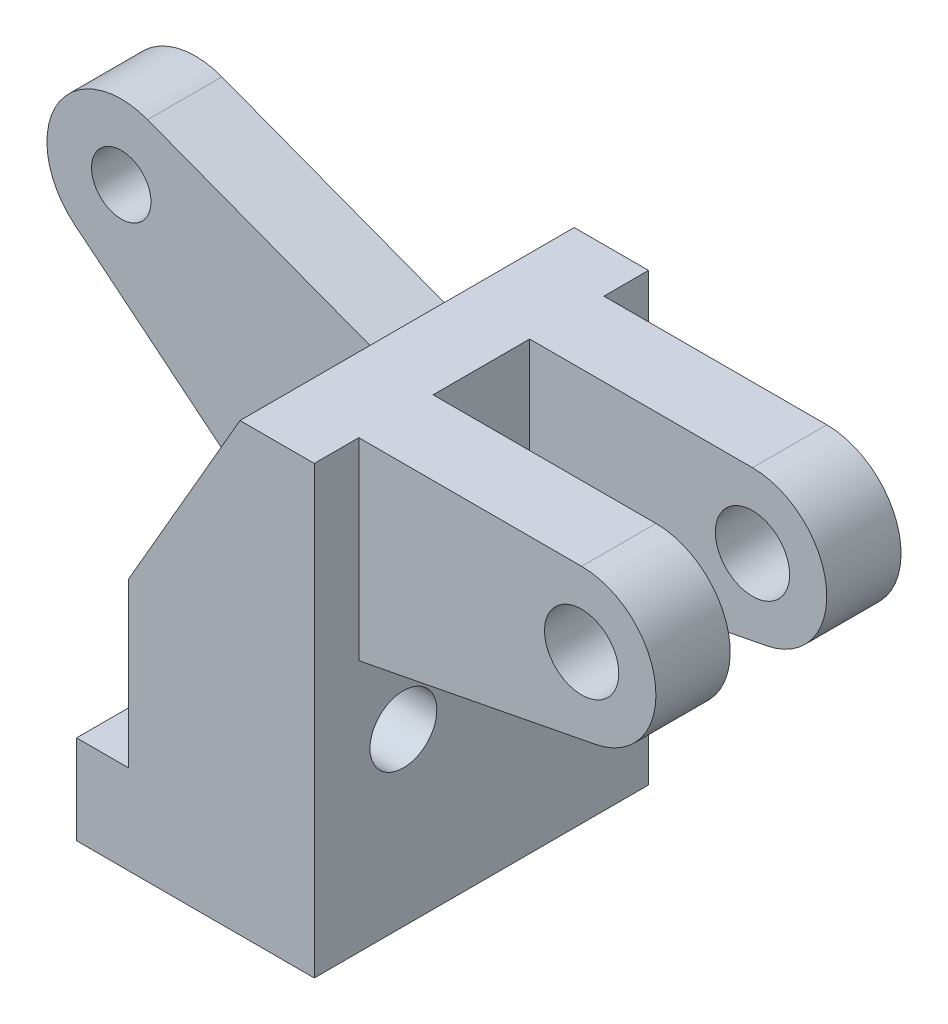
ISO-10303-21;
HEADER;
FILE_DESCRIPTION(('STEP AP214'),'2;1');
FILE_NAME('part.step','',(''),(''),'','','');
FILE_SCHEMA(('AUTOMOTIVE_DESIGN { 1 0 10303 214 1 1 1 1 }'));
ENDSEC;
DATA;
#1=APPLICATION_CONTEXT('core data for automotive mechanical design processes');
#2=APPLICATION_PROTOCOL_DEFINITION('international standard','automotive_design',2000,#1);
#3=PRODUCT_CONTEXT('',#1,'mechanical');
#4=PRODUCT('Part','Part','',(#3));
#5=PRODUCT_RELATED_PRODUCT_CATEGORY('part','',(#4));
#6=PRODUCT_DEFINITION_FORMATION('','',#4);
#7=PRODUCT_DEFINITION_CONTEXT('part definition',#1,'design');
#8=PRODUCT_DEFINITION('design','',#6,#7);
#9=PRODUCT_DEFINITION_SHAPE('','',#8);
#10=(LENGTH_UNIT() NAMED_UNIT(*) SI_UNIT(.MILLI.,.METRE.));
#11=(NAMED_UNIT(*) PLANE_ANGLE_UNIT() SI_UNIT($,.RADIAN.));
#12=(NAMED_UNIT(*) SI_UNIT($,.STERADIAN.) SOLID_ANGLE_UNIT());
#13=UNCERTAINTY_MEASURE_WITH_UNIT(LENGTH_MEASURE(1.E-05),#10,'distance_accuracy_value','');
#14=(GEOMETRIC_REPRESENTATION_CONTEXT(3) GLOBAL_UNCERTAINTY_ASSIGNED_CONTEXT((#13)) GLOBAL_UNIT_ASSIGNED_CONTEXT((#10,
#11,#12)) REPRESENTATION_CONTEXT('',''));
#15=CARTESIAN_POINT('',(0.,0.,0.));
#16=DIRECTION('',(0.,0.,1.));
#17=DIRECTION('',(1.,0.,0.));
#18=AXIS2_PLACEMENT_3D('',#15,#16,#17);
#19=CARTESIAN_POINT('',(30.,50.,-70.2074417675062));
#20=DIRECTION('',(0.,0.,1.));
#21=DIRECTION('',(1.,0.,0.));
#22=AXIS2_PLACEMENT_3D('',#19,#20,#21);
#23=CYLINDRICAL_SURFACE('',#22,10.);
#24=CARTESIAN_POINT('',(30.,50.,-6.50000000000001));
#25=DIRECTION('',(0.,0.,-1.));
#26=DIRECTION('',(-1.,0.,0.));
#27=AXIS2_PLACEMENT_3D('',#24,#25,#26);
#28=CIRCLE('',#27,10.);
#29=CARTESIAN_POINT('',(31.9025818157154,40.1826590955336,-6.50000000000001));
#30=VERTEX_POINT('',#29);
#31=CARTESIAN_POINT('',(30.,60.,-6.5));
#32=VERTEX_POINT('',#31);
#33=EDGE_CURVE('E253',#30,#32,#28,.F.);
#34=ORIENTED_EDGE('',*,*,#33,.F.);
#35=DIRECTION('',(0.,0.,1.));
#36=VECTOR('',#35,1.);
#37=CARTESIAN_POINT('',(31.9025818157154,40.1826590955336,-70.2074417675062));
#38=LINE('',#37,#36);
#39=CARTESIAN_POINT('',(31.9025818157154,40.1826590955336,-16.5));
#40=VERTEX_POINT('',#39);
#41=EDGE_CURVE('E275',#40,#30,#38,.T.);
#42=ORIENTED_EDGE('',*,*,#41,.F.);
#43=CARTESIAN_POINT('',(30.,50.,-16.5));
#44=DIRECTION('',(0.,0.,1.));
#45=DIRECTION('',(1.,0.,0.));
#46=AXIS2_PLACEMENT_3D('',#43,#44,#45);
#47=CIRCLE('',#46,10.);
#48=CARTESIAN_POINT('',(30.,60.,-16.5));
#49=VERTEX_POINT('',#48);
#50=EDGE_CURVE('E62',#49,#40,#47,.F.);
#51=ORIENTED_EDGE('',*,*,#50,.F.);
#52=DIRECTION('',(0.,0.,1.));
#53=VECTOR('',#52,1.);
#54=CARTESIAN_POINT('',(30.,60.,-70.2074417675062));
#55=LINE('',#54,#53);
#56=EDGE_CURVE('E270',#49,#32,#55,.T.);
#57=ORIENTED_EDGE('',*,*,#56,.T.);
#58=EDGE_LOOP('',(#34,#42,#51,#57));
#59=FACE_BOUND('',#58,.T.);
#60=ADVANCED_FACE('F39',(#59),#23,.T.);
#61=CARTESIAN_POINT('',(0.,34.,-70.2074417675062));
#62=DIRECTION('',(0.190258181571541,-0.98173409044664,0.));
#63=DIRECTION('',(0.98173409044664,0.190258181571541,0.));
#64=AXIS2_PLACEMENT_3D('',#61,#62,#63);
#65=PLANE('',#64);
#66=DIRECTION('',(0.98173409044664,0.190258181571541,0.));
#67=VECTOR('',#66,1.);
#68=CARTESIAN_POINT('',(0.,34.,-6.50000000000001));
#69=LINE('',#68,#67);
#70=CARTESIAN_POINT('',(0.,34.,-6.5));
#71=VERTEX_POINT('',#70);
#72=EDGE_CURVE('E249',#71,#30,#69,.T.);
#73=ORIENTED_EDGE('',*,*,#72,.F.);
#74=DIRECTION('',(0.,0.,1.));
#75=VECTOR('',#74,1.);
#76=CARTESIAN_POINT('',(0.,34.,-70.2074417675062));
#77=LINE('',#76,#75);
#78=CARTESIAN_POINT('',(0.,34.,-16.5));
#79=VERTEX_POINT('',#78);
#80=EDGE_CURVE('E268',#79,#71,#77,.T.);
#81=ORIENTED_EDGE('',*,*,#80,.F.);
#82=DIRECTION('',(-0.98173409044664,-0.190258181571541,0.));
#83=VECTOR('',#82,1.);
#84=CARTESIAN_POINT('',(0.,34.,-16.5));
#85=LINE('',#84,#83);
#86=EDGE_CURVE('E243',#40,#79,#85,.T.);
#87=ORIENTED_EDGE('',*,*,#86,.F.);
#88=ORIENTED_EDGE('',*,*,#41,.T.);
#89=EDGE_LOOP('',(#73,#81,#87,#88));
#90=FACE_BOUND('',#89,.T.);
#91=ADVANCED_FACE('F388',(#90),#65,.T.);
#92=CARTESIAN_POINT('',(-25.0111069989303,34.,22.5));
#93=DIRECTION('',(0.866025403784438,-0.500000000000001,0.));
#94=DIRECTION('',(0.500000000000001,0.866025403784438,0.));
#95=AXIS2_PLACEMENT_3D('',#92,#93,#94);
#96=PLANE('',#95);
#97=DIRECTION('',(0.500000000000001,0.866025403784438,0.));
#98=VECTOR('',#97,1.);
#99=CARTESIAN_POINT('',(-25.0111069989303,34.,5.));
#100=LINE('',#99,#98);
#101=CARTESIAN_POINT('',(-25.0111069989303,34.,5.00000000000001));
#102=VERTEX_POINT('',#101);
#103=CARTESIAN_POINT('',(-10.,60.,5.));
#104=VERTEX_POINT('',#103);
#105=EDGE_CURVE('E291',#102,#104,#100,.T.);
#106=ORIENTED_EDGE('',*,*,#105,.F.);
#107=DIRECTION('',(0.,0.,-1.));
#108=VECTOR('',#107,1.);
#109=CARTESIAN_POINT('',(-25.0111069989303,34.,22.5));
#110=LINE('',#109,#108);
#111=CARTESIAN_POINT('',(-25.0111069989303,34.,22.5));
#112=VERTEX_POINT('',#111);
#113=EDGE_CURVE('E231',#112,#102,#110,.T.);
#114=ORIENTED_EDGE('',*,*,#113,.F.);
#115=DIRECTION('',(-0.500000000000001,-0.866025403784438,0.));
#116=VECTOR('',#115,1.);
#117=CARTESIAN_POINT('',(-25.0111069989303,34.,22.5));
#118=LINE('',#117,#116);
#119=CARTESIAN_POINT('',(-10.,60.,22.5));
#120=VERTEX_POINT('',#119);
#121=EDGE_CURVE('E191',#120,#112,#118,.T.);
#122=ORIENTED_EDGE('',*,*,#121,.F.);
#123=DIRECTION('',(0.,0.,-1.));
#124=VECTOR('',#123,1.);
#125=CARTESIAN_POINT('',(-10.,60.,22.5));
#126=LINE('',#125,#124);
#127=EDGE_CURVE('E11',#120,#104,#126,.T.);
#128=ORIENTED_EDGE('',*,*,#127,.T.);
#129=EDGE_LOOP('',(#106,#114,#122,#128));
#130=FACE_BOUND('',#129,.T.);
#131=ADVANCED_FACE('F348',(#130),#96,.F.);
#132=CARTESIAN_POINT('',(0.,60.,22.5));
#133=DIRECTION('',(-1.,0.,0.));
#134=DIRECTION('',(0.,-1.,0.));
#135=AXIS2_PLACEMENT_3D('',#132,#133,#134);
#136=PLANE('',#135);
#137=CARTESIAN_POINT('',(0.,23.,-10.5));
#138=DIRECTION('',(-1.,0.,0.));
#139=DIRECTION('',(0.,-1.,0.));
#140=AXIS2_PLACEMENT_3D('',#137,#138,#139);
#141=CIRCLE('',#140,4.5);
#142=CARTESIAN_POINT('',(0.,18.5,-10.5));
#143=VERTEX_POINT('',#142);
#144=EDGE_CURVE('E279',#143,#143,#141,.F.);
#145=ORIENTED_EDGE('',*,*,#144,.F.);
#146=EDGE_LOOP('',(#145));
#147=FACE_BOUND('',#146,.T.);
#148=CARTESIAN_POINT('',(0.,23.,10.5));
#149=DIRECTION('',(-1.,0.,0.));
#150=DIRECTION('',(0.,-1.,0.));
#151=AXIS2_PLACEMENT_3D('',#148,#149,#150);
#152=CIRCLE('',#151,4.5);
#153=CARTESIAN_POINT('',(0.,18.5,10.5));
#154=VERTEX_POINT('',#153);
#155=EDGE_CURVE('E280',#154,#154,#152,.F.);
#156=ORIENTED_EDGE('',*,*,#155,.F.);
#157=EDGE_LOOP('',(#156));
#158=FACE_BOUND('',#157,.T.);
#159=CARTESIAN_POINT('',(0.,34.,6.5));
#160=VERTEX_POINT('',#159);
#161=CARTESIAN_POINT('',(0.,34.,16.5));
#162=VERTEX_POINT('',#161);
#163=EDGE_CURVE('E263',#160,#162,#77,.T.);
#164=ORIENTED_EDGE('',*,*,#163,.T.);
#165=DIRECTION('',(0.,1.,0.));
#166=VECTOR('',#165,1.);
#167=CARTESIAN_POINT('',(0.,0.,16.5));
#168=LINE('',#167,#166);
#169=CARTESIAN_POINT('',(0.,60.,16.5));
#170=VERTEX_POINT('',#169);
#171=EDGE_CURVE('E183',#162,#170,#168,.T.);
#172=ORIENTED_EDGE('',*,*,#171,.T.);
#173=DIRECTION('',(0.,0.,1.));
#174=VECTOR('',#173,1.);
#175=CARTESIAN_POINT('',(0.,60.,16.5));
#176=LINE('',#175,#174);
#177=CARTESIAN_POINT('',(0.,60.,22.5));
#178=VERTEX_POINT('',#177);
#179=EDGE_CURVE('E181',#170,#178,#176,.T.);
#180=ORIENTED_EDGE('',*,*,#179,.T.);
#181=DIRECTION('',(0.,1.,0.));
#182=VECTOR('',#181,1.);
#183=CARTESIAN_POINT('',(0.,60.,22.5));
#184=LINE('',#183,#182);
#185=CARTESIAN_POINT('',(0.,0.,22.5));
#186=VERTEX_POINT('',#185);
#187=EDGE_CURVE('E168',#186,#178,#184,.T.);
#188=ORIENTED_EDGE('',*,*,#187,.F.);
#189=DIRECTION('',(0.,0.,-1.));
#190=VECTOR('',#189,1.);
#191=CARTESIAN_POINT('',(0.,0.,22.5));
#192=LINE('',#191,#190);
#193=CARTESIAN_POINT('',(0.,0.,-22.5));
#194=VERTEX_POINT('',#193);
#195=EDGE_CURVE('E210',#186,#194,#192,.T.);
#196=ORIENTED_EDGE('',*,*,#195,.T.);
#197=DIRECTION('',(0.,1.,0.));
#198=VECTOR('',#197,1.);
#199=CARTESIAN_POINT('',(0.,60.,-22.5));
#200=LINE('',#199,#198);
#201=CARTESIAN_POINT('',(0.,60.,-22.5));
#202=VERTEX_POINT('',#201);
#203=EDGE_CURVE('E208',#194,#202,#200,.T.);
#204=ORIENTED_EDGE('',*,*,#203,.T.);
#205=DIRECTION('',(0.,0.,1.));
#206=VECTOR('',#205,1.);
#207=CARTESIAN_POINT('',(0.,60.,-16.5));
#208=LINE('',#207,#206);
#209=CARTESIAN_POINT('',(0.,60.,-16.5));
#210=VERTEX_POINT('',#209);
#211=EDGE_CURVE('E371',#202,#210,#208,.T.);
#212=ORIENTED_EDGE('',*,*,#211,.T.);
#213=DIRECTION('',(0.,1.,0.));
#214=VECTOR('',#213,1.);
#215=CARTESIAN_POINT('',(0.,0.,-16.5));
#216=LINE('',#215,#214);
#217=EDGE_CURVE('E440',#79,#210,#216,.T.);
#218=ORIENTED_EDGE('',*,*,#217,.F.);
#219=ORIENTED_EDGE('',*,*,#80,.T.);
#220=DIRECTION('',(0.,1.,0.));
#221=VECTOR('',#220,1.);
#222=CARTESIAN_POINT('',(0.,0.,-6.5));
#223=LINE('',#222,#221);
#224=CARTESIAN_POINT('',(0.,60.,-6.5));
#225=VERTEX_POINT('',#224);
#226=EDGE_CURVE('E189',#71,#225,#223,.T.);
#227=ORIENTED_EDGE('',*,*,#226,.T.);
#228=DIRECTION('',(0.,0.,1.));
#229=VECTOR('',#228,1.);
#230=CARTESIAN_POINT('',(0.,60.,6.5));
#231=LINE('',#230,#229);
#232=CARTESIAN_POINT('',(0.,60.,6.5));
#233=VERTEX_POINT('',#232);
#234=EDGE_CURVE('E430',#225,#233,#231,.T.);
#235=ORIENTED_EDGE('',*,*,#234,.T.);
#236=DIRECTION('',(0.,1.,0.));
#237=VECTOR('',#236,1.);
#238=CARTESIAN_POINT('',(0.,0.,6.5));
#239=LINE('',#238,#237);
#240=EDGE_CURVE('E424',#160,#233,#239,.T.);
#241=ORIENTED_EDGE('',*,*,#240,.F.);
#242=EDGE_LOOP('',(#164,#172,#180,#188,#196,#204,#212,#218,#219,#227,#235,#241));
#243=FACE_BOUND('',#242,.T.);
#244=ADVANCED_FACE('F41',(#147,#158,#243),#136,.F.);
#245=CARTESIAN_POINT('',(-10.,60.,22.5));
#246=DIRECTION('',(0.,-1.,0.));
#247=DIRECTION('',(0.,0.,-1.));
#248=AXIS2_PLACEMENT_3D('',#245,#246,#247);
#249=PLANE('',#248);
#250=DIRECTION('',(-1.,0.,0.));
#251=VECTOR('',#250,1.);
#252=CARTESIAN_POINT('',(-10.,60.,22.5));
#253=LINE('',#252,#251);
#254=EDGE_CURVE('E172',#178,#120,#253,.T.);
#255=ORIENTED_EDGE('',*,*,#254,.F.);
#256=ORIENTED_EDGE('',*,*,#179,.F.);
#257=DIRECTION('',(-1.,0.,0.));
#258=VECTOR('',#257,1.);
#259=CARTESIAN_POINT('',(0.,60.,16.5));
#260=LINE('',#259,#258);
#261=CARTESIAN_POINT('',(30.,60.,16.5));
#262=VERTEX_POINT('',#261);
#263=EDGE_CURVE('E187',#262,#170,#260,.T.);
#264=ORIENTED_EDGE('',*,*,#263,.F.);
#265=CARTESIAN_POINT('',(30.,60.,6.5));
#266=VERTEX_POINT('',#265);
#267=EDGE_CURVE('E262',#266,#262,#55,.T.);
#268=ORIENTED_EDGE('',*,*,#267,.F.);
#269=DIRECTION('',(1.,0.,0.));
#270=VECTOR('',#269,1.);
#271=CARTESIAN_POINT('',(0.,60.,6.5));
#272=LINE('',#271,#270);
#273=EDGE_CURVE('E433',#233,#266,#272,.T.);
#274=ORIENTED_EDGE('',*,*,#273,.F.);
#275=ORIENTED_EDGE('',*,*,#234,.F.);
#276=DIRECTION('',(-1.,0.,0.));
#277=VECTOR('',#276,1.);
#278=CARTESIAN_POINT('',(0.,60.,-6.5));
#279=LINE('',#278,#277);
#280=EDGE_CURVE('E427',#32,#225,#279,.T.);
#281=ORIENTED_EDGE('',*,*,#280,.F.);
#282=ORIENTED_EDGE('',*,*,#56,.F.);
#283=DIRECTION('',(1.,0.,0.));
#284=VECTOR('',#283,1.);
#285=CARTESIAN_POINT('',(0.,60.,-16.5));
#286=LINE('',#285,#284);
#287=EDGE_CURVE('E374',#210,#49,#286,.T.);
#288=ORIENTED_EDGE('',*,*,#287,.F.);
#289=ORIENTED_EDGE('',*,*,#211,.F.);
#290=DIRECTION('',(-1.,0.,0.));
#291=VECTOR('',#290,1.);
#292=CARTESIAN_POINT('',(-10.,60.,-22.5));
#293=LINE('',#292,#291);
#294=CARTESIAN_POINT('',(-10.,60.,-22.5));
#295=VERTEX_POINT('',#294);
#296=EDGE_CURVE('E209',#202,#295,#293,.T.);
#297=ORIENTED_EDGE('',*,*,#296,.T.);
#298=CARTESIAN_POINT('',(-10.,60.,-4.99999999999999));
#299=VERTEX_POINT('',#298);
#300=EDGE_CURVE('E48',#299,#295,#126,.T.);
#301=ORIENTED_EDGE('',*,*,#300,.F.);
#302=DIRECTION('',(0.,0.,-1.));
#303=VECTOR('',#302,1.);
#304=CARTESIAN_POINT('',(-10.,60.,5.));
#305=LINE('',#304,#303);
#306=EDGE_CURVE('E211',#104,#299,#305,.T.);
#307=ORIENTED_EDGE('',*,*,#306,.F.);
#308=ORIENTED_EDGE('',*,*,#127,.F.);
#309=EDGE_LOOP('',(#255,#256,#264,#268,#274,#275,#281,#282,#288,#289,#297,#301,#307,#308));
#310=FACE_BOUND('',#309,.T.);
#311=ADVANCED_FACE('F194',(#310),#249,.F.);
#312=CARTESIAN_POINT('',(-25.0111069989303,34.,-4.99999999999999));
#313=VERTEX_POINT('',#312);
#314=CARTESIAN_POINT('',(-25.0111069989303,34.,-22.5));
#315=VERTEX_POINT('',#314);
#316=EDGE_CURVE('E235',#313,#315,#110,.T.);
#317=ORIENTED_EDGE('',*,*,#316,.F.);
#318=DIRECTION('',(0.500000000000001,0.866025403784438,0.));
#319=VECTOR('',#318,1.);
#320=CARTESIAN_POINT('',(-25.0111069989303,34.,-5.));
#321=LINE('',#320,#319);
#322=EDGE_CURVE('E286',#313,#299,#321,.T.);
#323=ORIENTED_EDGE('',*,*,#322,.T.);
#324=ORIENTED_EDGE('',*,*,#300,.T.);
#325=DIRECTION('',(-0.500000000000001,-0.866025403784438,0.));
#326=VECTOR('',#325,1.);
#327=CARTESIAN_POINT('',(-25.0111069989303,34.,-22.5));
#328=LINE('',#327,#326);
#329=EDGE_CURVE('E213',#295,#315,#328,.T.);
#330=ORIENTED_EDGE('',*,*,#329,.T.);
#331=EDGE_LOOP('',(#317,#323,#324,#330));
#332=FACE_BOUND('',#331,.T.);
#333=ADVANCED_FACE('F377',(#332),#96,.F.);
#334=CARTESIAN_POINT('',(-25.0111069989303,12.,22.5));
#335=DIRECTION('',(1.,0.,0.));
#336=DIRECTION('',(0.,0.,-1.));
#337=AXIS2_PLACEMENT_3D('',#334,#335,#336);
#338=PLANE('',#337);
#339=CARTESIAN_POINT('',(-25.0111069989303,23.,10.5));
#340=DIRECTION('',(-1.,0.,0.));
#341=DIRECTION('',(0.,0.,1.));
#342=AXIS2_PLACEMENT_3D('',#339,#340,#341);
#343=CIRCLE('',#342,4.5);
#344=CARTESIAN_POINT('',(-25.0111069989303,23.,15.));
#345=VERTEX_POINT('',#344);
#346=EDGE_CURVE('E273',#345,#345,#343,.T.);
#347=ORIENTED_EDGE('',*,*,#346,.F.);
#348=EDGE_LOOP('',(#347));
#349=FACE_BOUND('',#348,.T.);
#350=CARTESIAN_POINT('',(-25.0111069989303,23.,-10.5));
#351=DIRECTION('',(-1.,0.,0.));
#352=DIRECTION('',(0.,0.,1.));
#353=AXIS2_PLACEMENT_3D('',#350,#351,#352);
#354=CIRCLE('',#353,4.5);
#355=CARTESIAN_POINT('',(-25.0111069989303,23.,-6.));
#356=VERTEX_POINT('',#355);
#357=EDGE_CURVE('E285',#356,#356,#354,.T.);
#358=ORIENTED_EDGE('',*,*,#357,.F.);
#359=EDGE_LOOP('',(#358));
#360=FACE_BOUND('',#359,.T.);
#361=DIRECTION('',(0.,-1.,0.));
#362=VECTOR('',#361,1.);
#363=CARTESIAN_POINT('',(-25.0111069989303,12.,-22.5));
#364=LINE('',#363,#362);
#365=CARTESIAN_POINT('',(-25.0111069989303,12.,-22.5));
#366=VERTEX_POINT('',#365);
#367=EDGE_CURVE('E216',#315,#366,#364,.T.);
#368=ORIENTED_EDGE('',*,*,#367,.T.);
#369=DIRECTION('',(0.,0.,-1.));
#370=VECTOR('',#369,1.);
#371=CARTESIAN_POINT('',(-25.0111069989303,12.,22.5));
#372=LINE('',#371,#370);
#373=CARTESIAN_POINT('',(-25.0111069989303,12.,22.5));
#374=VERTEX_POINT('',#373);
#375=EDGE_CURVE('E233',#374,#366,#372,.T.);
#376=ORIENTED_EDGE('',*,*,#375,.F.);
#377=DIRECTION('',(0.,-1.,0.));
#378=VECTOR('',#377,1.);
#379=CARTESIAN_POINT('',(-25.0111069989303,12.,22.5));
#380=LINE('',#379,#378);
#381=EDGE_CURVE('E197',#112,#374,#380,.T.);
#382=ORIENTED_EDGE('',*,*,#381,.F.);
#383=ORIENTED_EDGE('',*,*,#113,.T.);
#384=DIRECTION('',(0.,0.,-1.));
#385=VECTOR('',#384,1.);
#386=CARTESIAN_POINT('',(-25.0111069989303,34.,5.));
#387=LINE('',#386,#385);
#388=EDGE_CURVE('E305',#102,#313,#387,.T.);
#389=ORIENTED_EDGE('',*,*,#388,.T.);
#390=ORIENTED_EDGE('',*,*,#316,.T.);
#391=EDGE_LOOP('',(#368,#376,#382,#383,#389,#390));
#392=FACE_BOUND('',#391,.T.);
#393=ADVANCED_FACE('F351',(#349,#360,#392),#338,.F.);
#394=CARTESIAN_POINT('',(-32.,12.,22.5));
#395=DIRECTION('',(0.,-1.,0.));
#396=DIRECTION('',(0.,0.,-1.));
#397=AXIS2_PLACEMENT_3D('',#394,#395,#396);
#398=PLANE('',#397);
#399=DIRECTION('',(-1.,0.,0.));
#400=VECTOR('',#399,1.);
#401=CARTESIAN_POINT('',(-32.,12.,-22.5));
#402=LINE('',#401,#400);
#403=CARTESIAN_POINT('',(-32.,12.,-22.5));
#404=VERTEX_POINT('',#403);
#405=EDGE_CURVE('E217',#366,#404,#402,.T.);
#406=ORIENTED_EDGE('',*,*,#405,.T.);
#407=DIRECTION('',(0.,0.,-1.));
#408=VECTOR('',#407,1.);
#409=CARTESIAN_POINT('',(-32.,12.,22.5));
#410=LINE('',#409,#408);
#411=CARTESIAN_POINT('',(-32.,12.,22.5));
#412=VERTEX_POINT('',#411);
#413=EDGE_CURVE('E226',#412,#404,#410,.T.);
#414=ORIENTED_EDGE('',*,*,#413,.F.);
#415=DIRECTION('',(-1.,0.,0.));
#416=VECTOR('',#415,1.);
#417=CARTESIAN_POINT('',(-32.,12.,22.5));
#418=LINE('',#417,#416);
#419=EDGE_CURVE('E205',#374,#412,#418,.T.);
#420=ORIENTED_EDGE('',*,*,#419,.F.);
#421=ORIENTED_EDGE('',*,*,#375,.T.);
#422=EDGE_LOOP('',(#406,#414,#420,#421));
#423=FACE_BOUND('',#422,.T.);
#424=ADVANCED_FACE('F356',(#423),#398,.F.);
#425=CARTESIAN_POINT('',(-32.,0.,22.5));
#426=DIRECTION('',(1.,0.,0.));
#427=DIRECTION('',(0.,0.,-1.));
#428=AXIS2_PLACEMENT_3D('',#425,#426,#427);
#429=PLANE('',#428);
#430=DIRECTION('',(0.,-1.,0.));
#431=VECTOR('',#430,1.);
#432=CARTESIAN_POINT('',(-32.,0.,-22.5));
#433=LINE('',#432,#431);
#434=CARTESIAN_POINT('',(-32.,0.,-22.5));
#435=VERTEX_POINT('',#434);
#436=EDGE_CURVE('E219',#404,#435,#433,.T.);
#437=ORIENTED_EDGE('',*,*,#436,.T.);
#438=DIRECTION('',(0.,0.,-1.));
#439=VECTOR('',#438,1.);
#440=CARTESIAN_POINT('',(-32.,0.,22.5));
#441=LINE('',#440,#439);
#442=CARTESIAN_POINT('',(-32.,0.,22.5));
#443=VERTEX_POINT('',#442);
#444=EDGE_CURVE('E223',#443,#435,#441,.T.);
#445=ORIENTED_EDGE('',*,*,#444,.F.);
#446=DIRECTION('',(0.,-1.,0.));
#447=VECTOR('',#446,1.);
#448=CARTESIAN_POINT('',(-32.,0.,22.5));
#449=LINE('',#448,#447);
#450=EDGE_CURVE('E204',#412,#443,#449,.T.);
#451=ORIENTED_EDGE('',*,*,#450,.F.);
#452=ORIENTED_EDGE('',*,*,#413,.T.);
#453=EDGE_LOOP('',(#437,#445,#451,#452));
#454=FACE_BOUND('',#453,.T.);
#455=ADVANCED_FACE('F365',(#454),#429,.F.);
#456=CARTESIAN_POINT('',(0.,0.,22.5));
#457=DIRECTION('',(0.,1.,0.));
#458=DIRECTION('',(-1.,0.,0.));
#459=AXIS2_PLACEMENT_3D('',#456,#457,#458);
#460=PLANE('',#459);
#461=DIRECTION('',(1.,0.,0.));
#462=VECTOR('',#461,1.);
#463=CARTESIAN_POINT('',(0.,0.,-22.5));
#464=LINE('',#463,#462);
#465=EDGE_CURVE('E176',#435,#194,#464,.T.);
#466=ORIENTED_EDGE('',*,*,#465,.T.);
#467=ORIENTED_EDGE('',*,*,#195,.F.);
#468=DIRECTION('',(1.,0.,0.));
#469=VECTOR('',#468,1.);
#470=CARTESIAN_POINT('',(0.,0.,22.5));
#471=LINE('',#470,#469);
#472=EDGE_CURVE('E179',#443,#186,#471,.T.);
#473=ORIENTED_EDGE('',*,*,#472,.F.);
#474=ORIENTED_EDGE('',*,*,#444,.T.);
#475=EDGE_LOOP('',(#466,#467,#473,#474));
#476=FACE_BOUND('',#475,.T.);
#477=ADVANCED_FACE('F370',(#476),#460,.F.);
#478=CARTESIAN_POINT('',(0.,0.,22.5));
#479=DIRECTION('',(0.,0.,-1.));
#480=DIRECTION('',(-1.,0.,0.));
#481=AXIS2_PLACEMENT_3D('',#478,#479,#480);
#482=PLANE('',#481);
#483=ORIENTED_EDGE('',*,*,#187,.T.);
#484=ORIENTED_EDGE('',*,*,#254,.T.);
#485=ORIENTED_EDGE('',*,*,#121,.T.);
#486=ORIENTED_EDGE('',*,*,#381,.T.);
#487=ORIENTED_EDGE('',*,*,#419,.T.);
#488=ORIENTED_EDGE('',*,*,#450,.T.);
#489=ORIENTED_EDGE('',*,*,#472,.T.);
#490=EDGE_LOOP('',(#483,#484,#485,#486,#487,#488,#489));
#491=FACE_BOUND('',#490,.T.);
#492=ADVANCED_FACE('F175',(#491),#482,.F.);
#493=CARTESIAN_POINT('',(0.,0.,-22.5));
#494=DIRECTION('',(0.,0.,-1.));
#495=DIRECTION('',(-1.,0.,0.));
#496=AXIS2_PLACEMENT_3D('',#493,#494,#495);
#497=PLANE('',#496);
#498=ORIENTED_EDGE('',*,*,#296,.F.);
#499=ORIENTED_EDGE('',*,*,#203,.F.);
#500=ORIENTED_EDGE('',*,*,#465,.F.);
#501=ORIENTED_EDGE('',*,*,#436,.F.);
#502=ORIENTED_EDGE('',*,*,#405,.F.);
#503=ORIENTED_EDGE('',*,*,#367,.F.);
#504=ORIENTED_EDGE('',*,*,#329,.F.);
#505=EDGE_LOOP('',(#498,#499,#500,#501,#502,#503,#504));
#506=FACE_BOUND('',#505,.T.);
#507=ADVANCED_FACE('F380',(#506),#497,.T.);
#508=CARTESIAN_POINT('',(-43.4863156129983,62.,5.));
#509=DIRECTION('',(0.,0.,1.));
#510=DIRECTION('',(1.,0.,0.));
#511=AXIS2_PLACEMENT_3D('',#508,#509,#510);
#512=PLANE('',#511);
#513=ORIENTED_EDGE('',*,*,#105,.T.);
#514=DIRECTION('',(-0.935064725336491,0.354477022430781,0.));
#515=VECTOR('',#514,1.);
#516=CARTESIAN_POINT('',(-39.9415453886905,71.3506472533649,5.));
#517=LINE('',#516,#515);
#518=CARTESIAN_POINT('',(-39.9415453886905,71.3506472533649,5.));
#519=VERTEX_POINT('',#518);
#520=EDGE_CURVE('E298',#104,#519,#517,.T.);
#521=ORIENTED_EDGE('',*,*,#520,.T.);
#522=CARTESIAN_POINT('',(-43.4863156129983,62.,5.));
#523=DIRECTION('',(0.,0.,1.));
#524=DIRECTION('',(1.,0.,0.));
#525=AXIS2_PLACEMENT_3D('',#522,#523,#524);
#526=CIRCLE('',#525,9.99999999999999);
#527=CARTESIAN_POINT('',(-49.8118285640856,54.2548153084884,5.));
#528=VERTEX_POINT('',#527);
#529=EDGE_CURVE('E297',#519,#528,#526,.T.);
#530=ORIENTED_EDGE('',*,*,#529,.T.);
#531=DIRECTION('',(0.774518469151167,-0.632551295108732,0.));
#532=VECTOR('',#531,1.);
#533=CARTESIAN_POINT('',(-25.0111069989303,34.,5.));
#534=LINE('',#533,#532);
#535=EDGE_CURVE('E303',#528,#102,#534,.T.);
#536=ORIENTED_EDGE('',*,*,#535,.T.);
#537=EDGE_LOOP('',(#513,#521,#530,#536));
#538=FACE_BOUND('',#537,.T.);
#539=CARTESIAN_POINT('',(-43.4863156129983,62.,5.));
#540=DIRECTION('',(0.,0.,1.));
#541=DIRECTION('',(1.,0.,0.));
#542=AXIS2_PLACEMENT_3D('',#539,#540,#541);
#543=CIRCLE('',#542,4.00000000000001);
#544=CARTESIAN_POINT('',(-39.4863156129983,62.,5.));
#545=VERTEX_POINT('',#544);
#546=EDGE_CURVE('E289',#545,#545,#543,.T.);
#547=ORIENTED_EDGE('',*,*,#546,.F.);
#548=EDGE_LOOP('',(#547));
#549=FACE_BOUND('',#548,.T.);
#550=ADVANCED_FACE('F347',(#538,#549),#512,.T.);
#551=CARTESIAN_POINT('',(-43.4863156129983,62.,-5.));
#552=DIRECTION('',(0.,0.,1.));
#553=DIRECTION('',(1.,0.,0.));
#554=AXIS2_PLACEMENT_3D('',#551,#552,#553);
#555=PLANE('',#554);
#556=ORIENTED_EDGE('',*,*,#322,.F.);
#557=DIRECTION('',(0.774518469151167,-0.632551295108732,0.));
#558=VECTOR('',#557,1.);
#559=CARTESIAN_POINT('',(-25.0111069989303,34.,-5.));
#560=LINE('',#559,#558);
#561=CARTESIAN_POINT('',(-49.8118285640856,54.2548153084884,-5.));
#562=VERTEX_POINT('',#561);
#563=EDGE_CURVE('E300',#562,#313,#560,.T.);
#564=ORIENTED_EDGE('',*,*,#563,.F.);
#565=CARTESIAN_POINT('',(-43.4863156129983,62.,-5.));
#566=DIRECTION('',(0.,0.,1.));
#567=DIRECTION('',(1.,0.,0.));
#568=AXIS2_PLACEMENT_3D('',#565,#566,#567);
#569=CIRCLE('',#568,9.99999999999999);
#570=CARTESIAN_POINT('',(-39.9415453886905,71.3506472533649,-5.));
#571=VERTEX_POINT('',#570);
#572=EDGE_CURVE('E306',#571,#562,#569,.T.);
#573=ORIENTED_EDGE('',*,*,#572,.F.);
#574=DIRECTION('',(-0.935064725336491,0.354477022430781,0.));
#575=VECTOR('',#574,1.);
#576=CARTESIAN_POINT('',(-39.9415453886905,71.3506472533649,-5.));
#577=LINE('',#576,#575);
#578=EDGE_CURVE('E308',#299,#571,#577,.T.);
#579=ORIENTED_EDGE('',*,*,#578,.F.);
#580=EDGE_LOOP('',(#556,#564,#573,#579));
#581=FACE_BOUND('',#580,.T.);
#582=CARTESIAN_POINT('',(-43.4863156129983,62.,-5.));
#583=DIRECTION('',(0.,0.,1.));
#584=DIRECTION('',(1.,0.,0.));
#585=AXIS2_PLACEMENT_3D('',#582,#583,#584);
#586=CIRCLE('',#585,4.00000000000001);
#587=CARTESIAN_POINT('',(-39.4863156129983,62.,-5.));
#588=VERTEX_POINT('',#587);
#589=EDGE_CURVE('E283',#588,#588,#586,.T.);
#590=ORIENTED_EDGE('',*,*,#589,.T.);
#591=EDGE_LOOP('',(#590));
#592=FACE_BOUND('',#591,.T.);
#593=ADVANCED_FACE('F331',(#581,#592),#555,.F.);
#594=CARTESIAN_POINT('',(-39.9415453886905,71.3506472533649,5.));
#595=DIRECTION('',(-0.354477022430781,-0.935064725336491,0.));
#596=DIRECTION('',(0.935064725336491,-0.354477022430781,0.));
#597=AXIS2_PLACEMENT_3D('',#594,#595,#596);
#598=PLANE('',#597);
#599=ORIENTED_EDGE('',*,*,#578,.T.);
#600=DIRECTION('',(0.,0.,-1.));
#601=VECTOR('',#600,1.);
#602=CARTESIAN_POINT('',(-39.9415453886905,71.3506472533649,5.));
#603=LINE('',#602,#601);
#604=EDGE_CURVE('E320',#519,#571,#603,.T.);
#605=ORIENTED_EDGE('',*,*,#604,.F.);
#606=ORIENTED_EDGE('',*,*,#520,.F.);
#607=ORIENTED_EDGE('',*,*,#306,.T.);
#608=EDGE_LOOP('',(#599,#605,#606,#607));
#609=FACE_BOUND('',#608,.T.);
#610=ADVANCED_FACE('F325',(#609),#598,.F.);
#611=CARTESIAN_POINT('',(-43.4863156129983,62.,5.));
#612=DIRECTION('',(0.,0.,-1.));
#613=DIRECTION('',(-1.,0.,0.));
#614=AXIS2_PLACEMENT_3D('',#611,#612,#613);
#615=CYLINDRICAL_SURFACE('',#614,9.99999999999999);
#616=ORIENTED_EDGE('',*,*,#572,.T.);
#617=DIRECTION('',(0.,0.,-1.));
#618=VECTOR('',#617,1.);
#619=CARTESIAN_POINT('',(-49.8118285640856,54.2548153084884,5.));
#620=LINE('',#619,#618);
#621=EDGE_CURVE('E314',#528,#562,#620,.T.);
#622=ORIENTED_EDGE('',*,*,#621,.F.);
#623=ORIENTED_EDGE('',*,*,#529,.F.);
#624=ORIENTED_EDGE('',*,*,#604,.T.);
#625=EDGE_LOOP('',(#616,#622,#623,#624));
#626=FACE_BOUND('',#625,.T.);
#627=ADVANCED_FACE('F337',(#626),#615,.T.);
#628=CARTESIAN_POINT('',(-25.0111069989303,34.,5.));
#629=DIRECTION('',(0.632551295108732,0.774518469151167,0.));
#630=DIRECTION('',(-0.774518469151167,0.632551295108732,0.));
#631=AXIS2_PLACEMENT_3D('',#628,#629,#630);
#632=PLANE('',#631);
#633=ORIENTED_EDGE('',*,*,#563,.T.);
#634=ORIENTED_EDGE('',*,*,#388,.F.);
#635=ORIENTED_EDGE('',*,*,#535,.F.);
#636=ORIENTED_EDGE('',*,*,#621,.T.);
#637=EDGE_LOOP('',(#633,#634,#635,#636));
#638=FACE_BOUND('',#637,.T.);
#639=ADVANCED_FACE('F342',(#638),#632,.F.);
#640=CARTESIAN_POINT('',(-43.4863156129983,62.,5.));
#641=DIRECTION('',(0.,0.,-1.));
#642=DIRECTION('',(-1.,0.,0.));
#643=AXIS2_PLACEMENT_3D('',#640,#641,#642);
#644=CYLINDRICAL_SURFACE('',#643,4.00000000000001);
#645=ORIENTED_EDGE('',*,*,#546,.T.);
#646=EDGE_LOOP('',(#645));
#647=FACE_BOUND('',#646,.T.);
#648=ORIENTED_EDGE('',*,*,#589,.F.);
#649=EDGE_LOOP('',(#648));
#650=FACE_BOUND('',#649,.T.);
#651=ADVANCED_FACE('F480',(#647,#650),#644,.F.);
#652=CARTESIAN_POINT('',(0.001000000000001,23.,-10.5));
#653=DIRECTION('',(-1.,0.,0.));
#654=DIRECTION('',(0.,0.,1.));
#655=AXIS2_PLACEMENT_3D('',#652,#653,#654);
#656=CYLINDRICAL_SURFACE('',#655,4.5);
#657=ORIENTED_EDGE('',*,*,#357,.T.);
#658=EDGE_LOOP('',(#657));
#659=FACE_BOUND('',#658,.T.);
#660=ORIENTED_EDGE('',*,*,#144,.T.);
#661=EDGE_LOOP('',(#660));
#662=FACE_BOUND('',#661,.T.);
#663=ADVANCED_FACE('F413',(#659,#662),#656,.F.);
#664=CARTESIAN_POINT('',(0.001000000000001,23.,10.5));
#665=DIRECTION('',(-1.,0.,0.));
#666=DIRECTION('',(0.,0.,1.));
#667=AXIS2_PLACEMENT_3D('',#664,#665,#666);
#668=CYLINDRICAL_SURFACE('',#667,4.5);
#669=ORIENTED_EDGE('',*,*,#346,.T.);
#670=EDGE_LOOP('',(#669));
#671=FACE_BOUND('',#670,.T.);
#672=ORIENTED_EDGE('',*,*,#155,.T.);
#673=EDGE_LOOP('',(#672));
#674=FACE_BOUND('',#673,.T.);
#675=ADVANCED_FACE('F401',(#671,#674),#668,.F.);
#676=CARTESIAN_POINT('',(30.,50.,16.5));
#677=DIRECTION('',(0.,0.,-1.));
#678=DIRECTION('',(-1.,0.,0.));
#679=AXIS2_PLACEMENT_3D('',#676,#677,#678);
#680=CIRCLE('',#679,10.);
#681=CARTESIAN_POINT('',(31.9025818157154,40.1826590955336,16.5));
#682=VERTEX_POINT('',#681);
#683=EDGE_CURVE('E261',#682,#262,#680,.F.);
#684=ORIENTED_EDGE('',*,*,#683,.F.);
#685=CARTESIAN_POINT('',(31.9025818157154,40.1826590955336,6.50000000000001));
#686=VERTEX_POINT('',#685);
#687=EDGE_CURVE('E267',#686,#682,#38,.T.);
#688=ORIENTED_EDGE('',*,*,#687,.F.);
#689=CARTESIAN_POINT('',(30.,50.,6.50000000000001));
#690=DIRECTION('',(0.,0.,1.));
#691=DIRECTION('',(1.,0.,0.));
#692=AXIS2_PLACEMENT_3D('',#689,#690,#691);
#693=CIRCLE('',#692,10.);
#694=EDGE_CURVE('E57',#266,#686,#693,.F.);
#695=ORIENTED_EDGE('',*,*,#694,.F.);
#696=ORIENTED_EDGE('',*,*,#267,.T.);
#697=EDGE_LOOP('',(#684,#688,#695,#696));
#698=FACE_BOUND('',#697,.T.);
#699=ADVANCED_FACE('F392',(#698),#23,.T.);
#700=DIRECTION('',(0.98173409044664,0.190258181571541,0.));
#701=VECTOR('',#700,1.);
#702=CARTESIAN_POINT('',(0.,34.,16.5));
#703=LINE('',#702,#701);
#704=EDGE_CURVE('E256',#162,#682,#703,.T.);
#705=ORIENTED_EDGE('',*,*,#704,.F.);
#706=ORIENTED_EDGE('',*,*,#163,.F.);
#707=DIRECTION('',(-0.98173409044664,-0.190258181571541,0.));
#708=VECTOR('',#707,1.);
#709=CARTESIAN_POINT('',(0.,34.,6.50000000000001));
#710=LINE('',#709,#708);
#711=EDGE_CURVE('E242',#686,#160,#710,.T.);
#712=ORIENTED_EDGE('',*,*,#711,.F.);
#713=ORIENTED_EDGE('',*,*,#687,.T.);
#714=EDGE_LOOP('',(#705,#706,#712,#713));
#715=FACE_BOUND('',#714,.T.);
#716=ADVANCED_FACE('F396',(#715),#65,.T.);
#717=CARTESIAN_POINT('',(0.,0.,-16.5));
#718=DIRECTION('',(0.,0.,1.));
#719=DIRECTION('',(1.,0.,0.));
#720=AXIS2_PLACEMENT_3D('',#717,#718,#719);
#721=PLANE('',#720);
#722=ORIENTED_EDGE('',*,*,#50,.T.);
#723=ORIENTED_EDGE('',*,*,#86,.T.);
#724=ORIENTED_EDGE('',*,*,#217,.T.);
#725=ORIENTED_EDGE('',*,*,#287,.T.);
#726=EDGE_LOOP('',(#722,#723,#724,#725));
#727=FACE_BOUND('',#726,.T.);
#728=CARTESIAN_POINT('',(30.,50.,-16.5));
#729=DIRECTION('',(0.,0.,1.));
#730=DIRECTION('',(1.,0.,0.));
#731=AXIS2_PLACEMENT_3D('',#728,#729,#730);
#732=CIRCLE('',#731,4.99999999999999);
#733=CARTESIAN_POINT('',(35.,50.,-16.5));
#734=VERTEX_POINT('',#733);
#735=EDGE_CURVE('E236',#734,#734,#732,.F.);
#736=ORIENTED_EDGE('',*,*,#735,.F.);
#737=EDGE_LOOP('',(#736));
#738=FACE_BOUND('',#737,.T.);
#739=ADVANCED_FACE('F407',(#727,#738),#721,.F.);
#740=CARTESIAN_POINT('',(0.,0.,-6.5));
#741=DIRECTION('',(0.,0.,-1.));
#742=DIRECTION('',(-1.,0.,0.));
#743=AXIS2_PLACEMENT_3D('',#740,#741,#742);
#744=PLANE('',#743);
#745=ORIENTED_EDGE('',*,*,#33,.T.);
#746=ORIENTED_EDGE('',*,*,#280,.T.);
#747=ORIENTED_EDGE('',*,*,#226,.F.);
#748=ORIENTED_EDGE('',*,*,#72,.T.);
#749=EDGE_LOOP('',(#745,#746,#747,#748));
#750=FACE_BOUND('',#749,.T.);
#751=CARTESIAN_POINT('',(30.,50.,-6.50000000000001));
#752=DIRECTION('',(0.,0.,-1.));
#753=DIRECTION('',(-1.,0.,0.));
#754=AXIS2_PLACEMENT_3D('',#751,#752,#753);
#755=CIRCLE('',#754,4.99999999999999);
#756=CARTESIAN_POINT('',(35.,50.,-6.50000000000001));
#757=VERTEX_POINT('',#756);
#758=EDGE_CURVE('E244',#757,#757,#755,.F.);
#759=ORIENTED_EDGE('',*,*,#758,.F.);
#760=EDGE_LOOP('',(#759));
#761=FACE_BOUND('',#760,.T.);
#762=ADVANCED_FACE('F448',(#750,#761),#744,.F.);
#763=CARTESIAN_POINT('',(0.,0.,6.5));
#764=DIRECTION('',(0.,0.,1.));
#765=DIRECTION('',(1.,0.,0.));
#766=AXIS2_PLACEMENT_3D('',#763,#764,#765);
#767=PLANE('',#766);
#768=ORIENTED_EDGE('',*,*,#694,.T.);
#769=ORIENTED_EDGE('',*,*,#711,.T.);
#770=ORIENTED_EDGE('',*,*,#240,.T.);
#771=ORIENTED_EDGE('',*,*,#273,.T.);
#772=EDGE_LOOP('',(#768,#769,#770,#771));
#773=FACE_BOUND('',#772,.T.);
#774=CARTESIAN_POINT('',(30.,50.,6.50000000000001));
#775=DIRECTION('',(0.,0.,1.));
#776=DIRECTION('',(1.,0.,0.));
#777=AXIS2_PLACEMENT_3D('',#774,#775,#776);
#778=CIRCLE('',#777,4.99999999999999);
#779=CARTESIAN_POINT('',(35.,50.,6.50000000000001));
#780=VERTEX_POINT('',#779);
#781=EDGE_CURVE('E245',#780,#780,#778,.F.);
#782=ORIENTED_EDGE('',*,*,#781,.F.);
#783=EDGE_LOOP('',(#782));
#784=FACE_BOUND('',#783,.T.);
#785=ADVANCED_FACE('F425',(#773,#784),#767,.F.);
#786=CARTESIAN_POINT('',(0.,0.,16.5));
#787=DIRECTION('',(0.,0.,-1.));
#788=DIRECTION('',(-1.,0.,0.));
#789=AXIS2_PLACEMENT_3D('',#786,#787,#788);
#790=PLANE('',#789);
#791=ORIENTED_EDGE('',*,*,#683,.T.);
#792=ORIENTED_EDGE('',*,*,#263,.T.);
#793=ORIENTED_EDGE('',*,*,#171,.F.);
#794=ORIENTED_EDGE('',*,*,#704,.T.);
#795=EDGE_LOOP('',(#791,#792,#793,#794));
#796=FACE_BOUND('',#795,.T.);
#797=CARTESIAN_POINT('',(30.,50.,16.5));
#798=DIRECTION('',(0.,0.,-1.));
#799=DIRECTION('',(-1.,0.,0.));
#800=AXIS2_PLACEMENT_3D('',#797,#798,#799);
#801=CIRCLE('',#800,4.99999999999999);
#802=CARTESIAN_POINT('',(35.,50.,16.5));
#803=VERTEX_POINT('',#802);
#804=EDGE_CURVE('E43',#803,#803,#801,.F.);
#805=ORIENTED_EDGE('',*,*,#804,.F.);
#806=EDGE_LOOP('',(#805));
#807=FACE_BOUND('',#806,.T.);
#808=ADVANCED_FACE('F416',(#796,#807),#790,.F.);
#809=CARTESIAN_POINT('',(30.,50.,-70.2074417675062));
#810=DIRECTION('',(0.,0.,1.));
#811=DIRECTION('',(1.,0.,0.));
#812=AXIS2_PLACEMENT_3D('',#809,#810,#811);
#813=CYLINDRICAL_SURFACE('',#812,4.99999999999999);
#814=CARTESIAN_POINT('',(35.,50.,-6.50000000000001));
#815=CARTESIAN_POINT('',(35.,50.,-6.60416666666667));
#816=CARTESIAN_POINT('',(35.,50.,-6.70833333333333));
#817=CARTESIAN_POINT('',(35.,50.,-6.91666666666667));
#818=CARTESIAN_POINT('',(35.,50.,-7.02083333333334));
#819=CARTESIAN_POINT('',(35.,50.,-7.22916666666667));
#820=CARTESIAN_POINT('',(35.,50.,-7.33333333333333));
#821=CARTESIAN_POINT('',(35.,50.,-7.54166666666667));
#822=CARTESIAN_POINT('',(35.,50.,-7.64583333333334));
#823=CARTESIAN_POINT('',(35.,50.,-7.85416666666667));
#824=CARTESIAN_POINT('',(35.,50.,-7.95833333333334));
#825=CARTESIAN_POINT('',(35.,50.,-8.16666666666667));
#826=CARTESIAN_POINT('',(35.,50.,-8.27083333333334));
#827=CARTESIAN_POINT('',(35.,50.,-8.47916666666667));
#828=CARTESIAN_POINT('',(35.,50.,-8.58333333333334));
#829=CARTESIAN_POINT('',(35.,50.,-8.79166666666667));
#830=CARTESIAN_POINT('',(35.,50.,-8.89583333333334));
#831=CARTESIAN_POINT('',(35.,50.,-9.10416666666667));
#832=CARTESIAN_POINT('',(35.,50.,-9.20833333333334));
#833=CARTESIAN_POINT('',(35.,50.,-9.41666666666667));
#834=CARTESIAN_POINT('',(35.,50.,-9.52083333333333));
#835=CARTESIAN_POINT('',(35.,50.,-9.72916666666667));
#836=CARTESIAN_POINT('',(35.,50.,-9.83333333333333));
#837=CARTESIAN_POINT('',(35.,50.,-10.0416666666667));
#838=CARTESIAN_POINT('',(35.,50.,-10.1458333333333));
#839=CARTESIAN_POINT('',(35.,50.,-10.3541666666667));
#840=CARTESIAN_POINT('',(35.,50.,-10.4583333333333));
#841=CARTESIAN_POINT('',(35.,50.,-10.6666666666667));
#842=CARTESIAN_POINT('',(35.,50.,-10.7708333333333));
#843=CARTESIAN_POINT('',(35.,50.,-10.9791666666667));
#844=CARTESIAN_POINT('',(35.,50.,-11.0833333333333));
#845=CARTESIAN_POINT('',(35.,50.,-11.2916666666667));
#846=CARTESIAN_POINT('',(35.,50.,-11.3958333333333));
#847=CARTESIAN_POINT('',(35.,50.,-11.6041666666667));
#848=CARTESIAN_POINT('',(35.,50.,-11.7083333333333));
#849=CARTESIAN_POINT('',(35.,50.,-11.9166666666667));
#850=CARTESIAN_POINT('',(35.,50.,-12.0208333333333));
#851=CARTESIAN_POINT('',(35.,50.,-12.2291666666667));
#852=CARTESIAN_POINT('',(35.,50.,-12.3333333333333));
#853=CARTESIAN_POINT('',(35.,50.,-12.5416666666667));
#854=CARTESIAN_POINT('',(35.,50.,-12.6458333333333));
#855=CARTESIAN_POINT('',(35.,50.,-12.8541666666667));
#856=CARTESIAN_POINT('',(35.,50.,-12.9583333333333));
#857=CARTESIAN_POINT('',(35.,50.,-13.1666666666667));
#858=CARTESIAN_POINT('',(35.,50.,-13.2708333333333));
#859=CARTESIAN_POINT('',(35.,50.,-13.4791666666667));
#860=CARTESIAN_POINT('',(35.,50.,-13.5833333333333));
#861=CARTESIAN_POINT('',(35.,50.,-13.7916666666667));
#862=CARTESIAN_POINT('',(35.,50.,-13.8958333333333));
#863=CARTESIAN_POINT('',(35.,50.,-14.1041666666667));
#864=CARTESIAN_POINT('',(35.,50.,-14.2083333333333));
#865=CARTESIAN_POINT('',(35.,50.,-14.4166666666667));
#866=CARTESIAN_POINT('',(35.,50.,-14.5208333333333));
#867=CARTESIAN_POINT('',(35.,50.,-14.7291666666667));
#868=CARTESIAN_POINT('',(35.,50.,-14.8333333333333));
#869=CARTESIAN_POINT('',(35.,50.,-15.0416666666667));
#870=CARTESIAN_POINT('',(35.,50.,-15.1458333333333));
#871=CARTESIAN_POINT('',(35.,50.,-15.3541666666667));
#872=CARTESIAN_POINT('',(35.,50.,-15.4583333333333));
#873=CARTESIAN_POINT('',(35.,50.,-15.6666666666667));
#874=CARTESIAN_POINT('',(35.,50.,-15.7708333333333));
#875=CARTESIAN_POINT('',(35.,50.,-15.9791666666667));
#876=CARTESIAN_POINT('',(35.,50.,-16.0833333333333));
#877=CARTESIAN_POINT('',(35.,50.,-16.2916666666667));
#878=CARTESIAN_POINT('',(35.,50.,-16.3958333333333));
#879=CARTESIAN_POINT('',(35.,50.,-16.5));
#880=B_SPLINE_CURVE_WITH_KNOTS('',3,(#814,#815,#816,#817,#818,#819,#820,#821,#822,#823,#824,
#825,#826,#827,#828,#829,#830,#831,#832,#833,#834,#835,#836,#837,#838,#839,#840,#841,#842,#843,
#844,#845,#846,#847,#848,#849,#850,#851,#852,#853,#854,#855,#856,#857,#858,#859,#860,#861,#862,
#863,#864,#865,#866,#867,#868,#869,#870,#871,#872,#873,#874,#875,#876,#877,#878,#879),
.UNSPECIFIED.,.F.,.F.,(4,2,2,2,2,2,2,2,2,2,2,2,2,2,2,2,2,2,2,2,2,2,2,2,2,2,2,2,2,2,2,2,4),(0.,
0.312499999999993,0.625000000000001,0.937499999999994,1.25,1.5625,1.875,2.1875,2.5,2.8125,3.125,
3.4375,3.75,4.0625,4.375,4.6875,5.,5.3125,5.625,5.9375,6.25,6.5625,6.875,7.1875,
7.49999999999999,7.8125,8.12499999999999,8.43749999999999,8.74999999999999,9.06249999999999,
9.37499999999999,9.68749999999999,9.99999999999999),.UNSPECIFIED.);
#881=EDGE_CURVE('BSEAM462',#757,#734,#880,.T.);
#882=ORIENTED_EDGE('',*,*,#758,.T.);
#883=ORIENTED_EDGE('',*,*,#735,.T.);
#884=ORIENTED_EDGE('',*,*,#881,.T.);
#885=ORIENTED_EDGE('',*,*,#881,.F.);
#886=EDGE_LOOP('',(#882,#884,#883,#885));
#887=FACE_BOUND('',#886,.T.);
#888=ADVANCED_FACE('F462',(#887),#813,.F.);
#889=CARTESIAN_POINT('',(35.,50.,16.5));
#890=CARTESIAN_POINT('',(35.,50.,16.3958333333333));
#891=CARTESIAN_POINT('',(35.,50.,16.2916666666667));
#892=CARTESIAN_POINT('',(35.,50.,16.0833333333334));
#893=CARTESIAN_POINT('',(35.,50.,15.9791666666667));
#894=CARTESIAN_POINT('',(35.,50.,15.7708333333333));
#895=CARTESIAN_POINT('',(35.,50.,15.6666666666667));
#896=CARTESIAN_POINT('',(35.,50.,15.4583333333333));
#897=CARTESIAN_POINT('',(35.,50.,15.3541666666667));
#898=CARTESIAN_POINT('',(35.,50.,15.1458333333333));
#899=CARTESIAN_POINT('',(35.,50.,15.0416666666667));
#900=CARTESIAN_POINT('',(35.,50.,14.8333333333334));
#901=CARTESIAN_POINT('',(35.,50.,14.7291666666667));
#902=CARTESIAN_POINT('',(35.,50.,14.5208333333333));
#903=CARTESIAN_POINT('',(35.,50.,14.4166666666667));
#904=CARTESIAN_POINT('',(35.,50.,14.2083333333333));
#905=CARTESIAN_POINT('',(35.,50.,14.1041666666667));
#906=CARTESIAN_POINT('',(35.,50.,13.8958333333333));
#907=CARTESIAN_POINT('',(35.,50.,13.7916666666667));
#908=CARTESIAN_POINT('',(35.,50.,13.5833333333333));
#909=CARTESIAN_POINT('',(35.,50.,13.4791666666667));
#910=CARTESIAN_POINT('',(35.,50.,13.2708333333333));
#911=CARTESIAN_POINT('',(35.,50.,13.1666666666667));
#912=CARTESIAN_POINT('',(35.,50.,12.9583333333333));
#913=CARTESIAN_POINT('',(35.,50.,12.8541666666667));
#914=CARTESIAN_POINT('',(35.,50.,12.6458333333333));
#915=CARTESIAN_POINT('',(35.,50.,12.5416666666667));
#916=CARTESIAN_POINT('',(35.,50.,12.3333333333333));
#917=CARTESIAN_POINT('',(35.,50.,12.2291666666667));
#918=CARTESIAN_POINT('',(35.,50.,12.0208333333333));
#919=CARTESIAN_POINT('',(35.,50.,11.9166666666667));
#920=CARTESIAN_POINT('',(35.,50.,11.7083333333333));
#921=CARTESIAN_POINT('',(35.,50.,11.6041666666667));
#922=CARTESIAN_POINT('',(35.,50.,11.3958333333333));
#923=CARTESIAN_POINT('',(35.,50.,11.2916666666667));
#924=CARTESIAN_POINT('',(35.,50.,11.0833333333333));
#925=CARTESIAN_POINT('',(35.,50.,10.9791666666667));
#926=CARTESIAN_POINT('',(35.,50.,10.7708333333333));
#927=CARTESIAN_POINT('',(35.,50.,10.6666666666667));
#928=CARTESIAN_POINT('',(35.,50.,10.4583333333333));
#929=CARTESIAN_POINT('',(35.,50.,10.3541666666667));
#930=CARTESIAN_POINT('',(35.,50.,10.1458333333333));
#931=CARTESIAN_POINT('',(35.,50.,10.0416666666667));
#932=CARTESIAN_POINT('',(35.,50.,9.83333333333335));
#933=CARTESIAN_POINT('',(35.,50.,9.72916666666668));
#934=CARTESIAN_POINT('',(35.,50.,9.52083333333334));
#935=CARTESIAN_POINT('',(35.,50.,9.41666666666667));
#936=CARTESIAN_POINT('',(35.,50.,9.20833333333334));
#937=CARTESIAN_POINT('',(35.,50.,9.10416666666667));
#938=CARTESIAN_POINT('',(35.,50.,8.89583333333334));
#939=CARTESIAN_POINT('',(35.,50.,8.79166666666668));
#940=CARTESIAN_POINT('',(35.,50.,8.58333333333335));
#941=CARTESIAN_POINT('',(35.,50.,8.47916666666668));
#942=CARTESIAN_POINT('',(35.,50.,8.27083333333334));
#943=CARTESIAN_POINT('',(35.,50.,8.16666666666667));
#944=CARTESIAN_POINT('',(35.,50.,7.95833333333334));
#945=CARTESIAN_POINT('',(35.,50.,7.85416666666667));
#946=CARTESIAN_POINT('',(35.,50.,7.64583333333334));
#947=CARTESIAN_POINT('',(35.,50.,7.54166666666668));
#948=CARTESIAN_POINT('',(35.,50.,7.33333333333334));
#949=CARTESIAN_POINT('',(35.,50.,7.22916666666667));
#950=CARTESIAN_POINT('',(35.,50.,7.02083333333334));
#951=CARTESIAN_POINT('',(35.,50.,6.91666666666667));
#952=CARTESIAN_POINT('',(35.,50.,6.70833333333333));
#953=CARTESIAN_POINT('',(35.,50.,6.60416666666667));
#954=CARTESIAN_POINT('',(35.,50.,6.50000000000001));
#955=B_SPLINE_CURVE_WITH_KNOTS('',3,(#889,#890,#891,#892,#893,#894,#895,#896,#897,#898,#899,
#900,#901,#902,#903,#904,#905,#906,#907,#908,#909,#910,#911,#912,#913,#914,#915,#916,#917,#918,
#919,#920,#921,#922,#923,#924,#925,#926,#927,#928,#929,#930,#931,#932,#933,#934,#935,#936,#937,
#938,#939,#940,#941,#942,#943,#944,#945,#946,#947,#948,#949,#950,#951,#952,#953,#954),
.UNSPECIFIED.,.F.,.F.,(4,2,2,2,2,2,2,2,2,2,2,2,2,2,2,2,2,2,2,2,2,2,2,2,2,2,2,2,2,2,2,2,4),(0.,
0.312499999999993,0.625000000000001,0.937500000000008,1.25,1.56249999999999,1.875,
2.18750000000001,2.5,2.8125,3.125,3.43750000000001,3.75,4.0625,4.375,4.68750000000001,5.,5.3125,
5.62500000000001,5.93750000000001,6.25000000000001,6.5625,6.87500000000001,7.18750000000001,
7.50000000000001,7.8125,8.12500000000001,8.43750000000001,8.75000000000001,9.0625,
9.37500000000001,9.68750000000002,10.),.UNSPECIFIED.);
#956=EDGE_CURVE('BSEAM467',#803,#780,#955,.T.);
#957=ORIENTED_EDGE('',*,*,#804,.T.);
#958=ORIENTED_EDGE('',*,*,#781,.T.);
#959=ORIENTED_EDGE('',*,*,#956,.T.);
#960=ORIENTED_EDGE('',*,*,#956,.F.);
#961=EDGE_LOOP('',(#957,#959,#958,#960));
#962=FACE_BOUND('',#961,.T.);
#963=ADVANCED_FACE('F467',(#962),#813,.F.);
#964=CLOSED_SHELL('',(#60,#91,#131,#244,#311,#333,#393,#424,#455,#477,#492,#507,#550,#593,#610,
#627,#639,#651,#663,#675,#699,#716,#739,#762,#785,#808,#888,#963));
#965=MANIFOLD_SOLID_BREP('B2',#964);
#966=ADVANCED_BREP_SHAPE_REPRESENTATION('',(#18,#965),#14);
#967=SHAPE_DEFINITION_REPRESENTATION(#9,#966);
ENDSEC;
END-ISO-10303-21;
